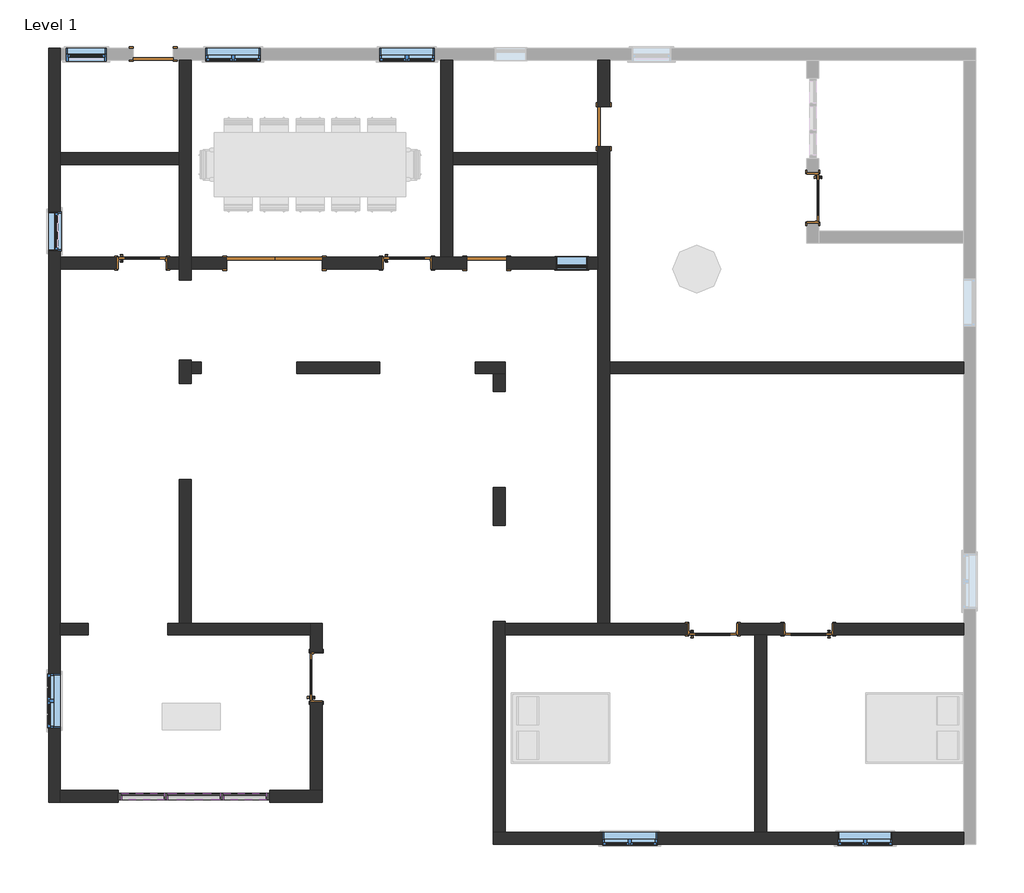
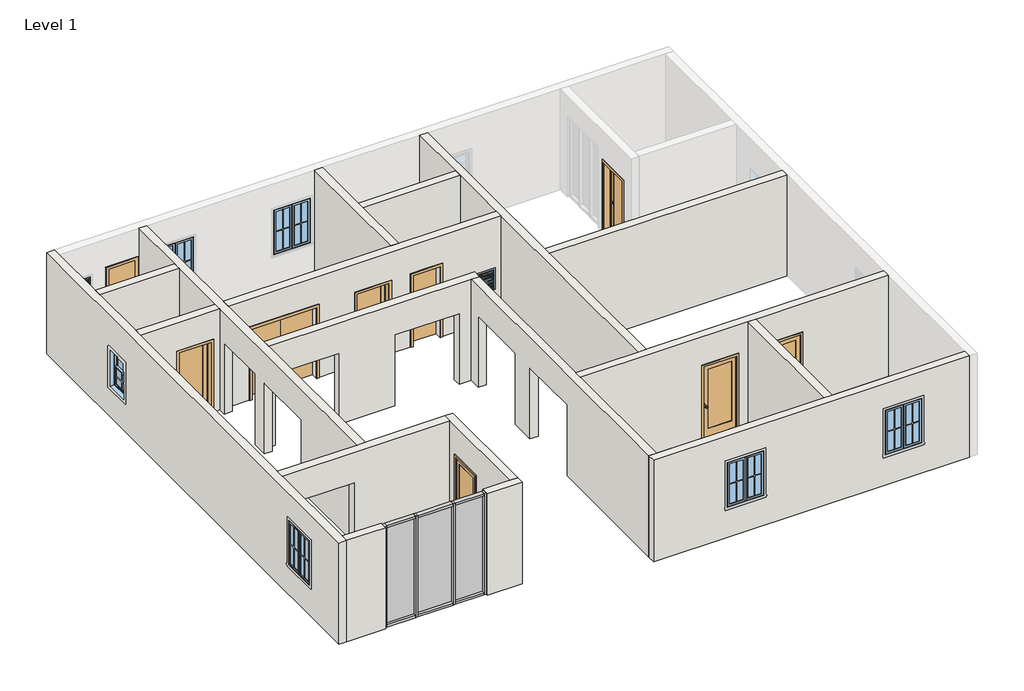
# One storey, part 1 of 2: 16 walls, 10 doors, 10 members, 8 windows, 3 plates.
"""IFC4 building model written with IfcOpenShell, lengths in millimetres."""

from ifc_helpers import new_model, si_unit, origin, origin_with_axes, place, context, project, spatial, polyline, outline, extrude, faceted_brep, transform, mapped, element, save
from components import door_963c5960, door_868ee8a9, door_3b97b8e7, door_5e1232af, member_c17f1be2, member_eaba9652, member_cfcad22e, member_3f395ae9, system_panel_glazed_52d31088, system_panel_glazed_62014e10, window_c95ebb39, window_d400040f, window_f2d8fef0

model = new_model("IFC4")

# Units and contexts
model_context = context("Model", 3, world=origin())
ifc_project = project(units=[si_unit("LENGTHUNIT", "METRE", prefix="MILLI")], contexts=[model_context])

# Site, building, storey
site = spatial("IfcSite", under=ifc_project)
building = spatial("IfcBuilding", under=site)
storey = spatial("IfcBuildingStorey", under=building, Name="Level 1", Elevation=0.0)

# Doors
placement = place(None, origin())
door_shape = door_963c5960(model_context)
element("IfcDoor", 1, ObjectType="Door-Double-Flush_Panel : 72\" x 84\"", at=placement, inside=storey, context=model_context, shape_type="MappedRepresentation", body=[
    mapped(door_shape, transform((-10733.2597103, 6532.3761524, 0.0), x_axis=(1.0, 0.0, 0.0), y_axis=(0.0, 1.0, 0.0), z_axis=(0.0, 0.0, 1.0))),
])
door_2_shape = door_868ee8a9(model_context)
element("IfcDoor", 2, ObjectType="Door-Interior-Single-1_Panel-Wood : 36\" x 84\"", at=placement, inside=storey, context=model_context, shape_type="MappedRepresentation", body=[
    mapped(door_2_shape, transform((-2354.8811947, -470.7808788, 0.0), x_axis=(1.0, 0.0, 0.0), y_axis=(0.0, 1.0, 0.0), z_axis=(0.0, 0.0, 1.0))),
])
door_3_shape = door_3b97b8e7(model_context)
element("IfcDoor", 3, ObjectType="Door-Interior-Single-1_Panel-Wood : 36\" x 84\"", at=placement, inside=storey, context=model_context, shape_type="MappedRepresentation", body=[
    mapped(door_3_shape, transform((-526.0811947, -470.7808788, 0.0), x_axis=(-1.0, 0.0, 0.0), y_axis=(0.0, -1.0, 0.0), z_axis=(0.0, 0.0, 1.0))),
])
element("IfcDoor", 4, ObjectType="Door-Interior-Single-1_Panel-Wood : 36\" x 84\"", at=placement, inside=storey, context=model_context, shape_type="MappedRepresentation", body=[
    mapped(door_3_shape, transform((-9943.6272884, -1382.0058788, 0.0), x_axis=(0.0, 1.0, 0.0), y_axis=(-1.0, 0.0, 0.0), z_axis=(0.0, 0.0, 1.0))),
])
element("IfcDoor", 5, ObjectType="Door-Interior-Single-1_Panel-Wood : 36\" x 84\"", at=placement, inside=storey, context=model_context, shape_type="MappedRepresentation", body=[
    mapped(door_3_shape, transform((-13264.0819759, 6535.5511524, 0.0), x_axis=(1.0, 0.0, 0.0), y_axis=(0.0, 1.0, 0.0), z_axis=(0.0, 0.0, 1.0))),
])
element("IfcDoor", 6, ObjectType="Door-Interior-Single-1_Panel-Wood : 36\" x 84\"", at=placement, inside=storey, context=model_context, shape_type="MappedRepresentation", body=[
    mapped(door_3_shape, transform((-8202.4374447, 6535.5511524, 0.0), x_axis=(1.0, 0.0, 0.0), y_axis=(0.0, 1.0, 0.0), z_axis=(0.0, 0.0, 1.0))),
])
element("IfcDoor", 7, ObjectType="Door-Interior-Single-1_Panel-Wood : 36\" x 84\"", at=placement, inside=storey, context=model_context, shape_type="MappedRepresentation", body=[
    mapped(door_3_shape, transform((-437.2804134, 7782.3835743, 0.0), x_axis=(0.0, -1.0, 0.0), y_axis=(1.0, 0.0, 0.0), z_axis=(0.0, 0.0, 1.0))),
])
door_4_shape = door_5e1232af(model_context)
element("IfcDoor", 8, ObjectType="Single-Flush : 30\" x 84\"", at=placement, inside=storey, context=model_context, shape_type="MappedRepresentation", body=[
    mapped(door_4_shape, transform((-13050.0671322, 10532.4792774, 0.0), x_axis=(1.0, 0.0, 0.0), y_axis=(0.0, 1.0, 0.0), z_axis=(0.0, 0.0, 1.0))),
])
element("IfcDoor", 9, ObjectType="Single-Flush : 30\" x 84\"", at=placement, inside=storey, context=model_context, shape_type="MappedRepresentation", body=[
    mapped(door_4_shape, transform((-4440.4593197, 9142.0277149, 0.0), x_axis=(0.0, -1.0, 0.0), y_axis=(1.0, 0.0, 0.0), z_axis=(0.0, 0.0, 1.0))),
])
element("IfcDoor", 10, ObjectType="Single-Flush : 30\" x 84\"", at=placement, inside=storey, context=model_context, shape_type="MappedRepresentation", body=[
    mapped(door_4_shape, transform((-6678.4374447, 6532.3761524, 0.0), x_axis=(-1.0, 0.0, 0.0), y_axis=(0.0, -1.0, 0.0), z_axis=(0.0, 0.0, 1.0))),
])

# Members
member_shape = member_c17f1be2(model_context)
element("IfcMember", 11, ObjectType="Rectangular Mullion : 2.5\" x 5\" rectangular", at=placement, inside=storey, context=model_context, shape_type="MappedRepresentation", body=[
    mapped(member_shape, transform((-10889.1819759, -3667.6090038, 3048.0), x_axis=(0.0, 0.0, 1.0), y_axis=(0.0, -1.0, 0.0), z_axis=(1.0, 0.0, 0.0))),
])
element("IfcMember", 12, ObjectType="Rectangular Mullion : 2.5\" x 5\" rectangular", at=placement, inside=storey, context=model_context, shape_type="MappedRepresentation", body=[
    mapped(member_shape, transform((-12838.6319759, -3667.6090038, 3048.0), x_axis=(0.0, 0.0, 1.0), y_axis=(0.0, -1.0, 0.0), z_axis=(1.0, 0.0, 0.0))),
])
element("IfcMember", 13, ObjectType="Rectangular Mullion : 2.5\" x 5\" rectangular", at=placement, inside=storey, context=model_context, shape_type="MappedRepresentation", body=[
    mapped(member_shape, transform((-13657.7819759, -3667.6090038, 0.0), x_axis=(0.0, 0.0, -1.0), y_axis=(0.0, -1.0, 0.0), z_axis=(-1.0, 0.0, 0.0))),
])
element("IfcMember", 14, ObjectType="Rectangular Mullion : 2.5\" x 5\" rectangular", at=placement, inside=storey, context=model_context, shape_type="MappedRepresentation", body=[
    mapped(member_shape, transform((-11708.3319759, -3667.6090038, 0.0), x_axis=(0.0, 0.0, -1.0), y_axis=(0.0, -1.0, 0.0), z_axis=(-1.0, 0.0, 0.0))),
])
member_2_shape = member_eaba9652(model_context)
element("IfcMember", 15, ObjectType="Rectangular Mullion : 2.5\" x 5\" rectangular", at=placement, inside=storey, context=model_context, shape_type="MappedRepresentation", body=[
    mapped(member_2_shape, transform((-12806.8819759, -3667.6090038, 0.0), x_axis=(1.0, 0.0, 0.0), y_axis=(0.0, -1.0, 0.0), z_axis=(0.0, 0.0, -1.0))),
])
element("IfcMember", 16, ObjectType="Rectangular Mullion : 2.5\" x 5\" rectangular", at=placement, inside=storey, context=model_context, shape_type="MappedRepresentation", body=[
    mapped(member_2_shape, transform((-11740.0819759, -3667.6090038, 0.0), x_axis=(1.0, 0.0, 0.0), y_axis=(0.0, -1.0, 0.0), z_axis=(0.0, 0.0, -1.0))),
])
member_3_shape = member_cfcad22e(model_context)
element("IfcMember", 17, ObjectType="Rectangular Mullion : 2.5\" x 5\" rectangular", at=placement, inside=storey, context=model_context, shape_type="MappedRepresentation", body=[
    mapped(member_3_shape, transform((-12775.1319759, -3667.6090038, 0.0), x_axis=(0.0, 0.0, -1.0), y_axis=(0.0, -1.0, 0.0), z_axis=(-1.0, 0.0, 0.0))),
])
element("IfcMember", 18, ObjectType="Rectangular Mullion : 2.5\" x 5\" rectangular", at=placement, inside=storey, context=model_context, shape_type="MappedRepresentation", body=[
    mapped(member_3_shape, transform((-11771.8319759, -3667.6090038, 3048.0), x_axis=(0.0, 0.0, 1.0), y_axis=(0.0, -1.0, 0.0), z_axis=(1.0, 0.0, 0.0))),
])
member_4_shape = member_3f395ae9(model_context)
element("IfcMember", 19, ObjectType="Rectangular Mullion : 2.5\" x 5\" rectangular", at=placement, inside=storey, context=model_context, shape_type="MappedRepresentation", body=[
    mapped(member_4_shape, transform((-13721.2819759, -3667.6090038, 3048.0), x_axis=(-1.0, 0.0, 0.0), y_axis=(0.0, -1.0, 0.0), z_axis=(0.0, 0.0, 1.0))),
])
element("IfcMember", 20, ObjectType="Rectangular Mullion : 2.5\" x 5\" rectangular", at=placement, inside=storey, context=model_context, shape_type="MappedRepresentation", body=[
    mapped(member_4_shape, transform((-10825.6819759, -3667.6090038, 0.0), x_axis=(1.0, 0.0, 0.0), y_axis=(0.0, -1.0, 0.0), z_axis=(0.0, 0.0, -1.0))),
])

# Plates
system_panel_glazed_shape = system_panel_glazed_52d31088(model_context)
element("IfcPlate", 21, ObjectType="System Panel : Glazed", at=placement, inside=storey, context=model_context, shape_type="MappedRepresentation", body=[
    mapped(system_panel_glazed_shape, transform((-13248.2069759, -3667.6090038, 63.5), x_axis=(1.0, 0.0, 0.0), y_axis=(0.0, 1.0, 0.0), z_axis=(0.0, 0.0, 1.0))),
])
element("IfcPlate", 22, ObjectType="System Panel : Glazed", at=placement, inside=storey, context=model_context, shape_type="MappedRepresentation", body=[
    mapped(system_panel_glazed_shape, transform((-11298.7569759, -3667.6090038, 63.5), x_axis=(1.0, 0.0, 0.0), y_axis=(0.0, 1.0, 0.0), z_axis=(0.0, 0.0, 1.0))),
])
system_panel_glazed_2_shape = system_panel_glazed_62014e10(model_context)
element("IfcPlate", 23, ObjectType="System Panel : Glazed", at=placement, inside=storey, context=model_context, shape_type="MappedRepresentation", body=[
    mapped(system_panel_glazed_2_shape, transform((-12273.4819759, -3667.6090038, 63.5), x_axis=(1.0, 0.0, 0.0), y_axis=(0.0, 1.0, 0.0), z_axis=(0.0, 0.0, 1.0))),
])

# Walls
element("IfcWall", 24, ObjectType="9\" wall", at=placement, inside=storey, context=model_context, shape_type="Brep", body=[
    faceted_brep([(-15054.7819759, 10646.7792774, 0.0), (-15054.7819759, -3781.9090038, 0.0), (-15054.7819759, -3781.9090038, 3048.0), (-15054.7819759, 10646.7792774, 3048.0), (-15054.7819759, -1318.5058788, 2260.6), (-15054.7819759, -2359.9058788, 2260.6), (-15054.7819759, -2359.9058788, 914.4), (-15054.7819759, -1318.5058788, 914.4), (-15054.7819759, 7522.9761524, 2082.8), (-15054.7819759, 6760.9761524, 2082.8), (-15054.7819759, 6760.9761524, 914.4), (-15054.7819759, 7522.9761524, 914.4), (-14826.1819759, 10646.7792774, 0.0), (-14826.1819759, 10646.7792774, 3048.0), (-14826.1819759, 10418.1792774, 3048.0), (-14826.1819759, 8646.6284962, 3048.0), (-14826.1819759, 8418.0284962, 3048.0), (-14826.1819759, 6646.6761524, 3048.0), (-14826.1819759, 6418.0761524, 3048.0), (-14826.1819759, -353.3058788, 3048.0), (-14826.1819759, -581.9058788, 3048.0), (-14826.1819759, -3553.3090038, 3048.0), (-14826.1819759, -3781.9090038, 3048.0), (-14826.1819759, -3781.9090038, 0.0), (-14826.1819759, -3553.3090038, 0.0), (-14826.1819759, -581.9058788, 0.0), (-14826.1819759, -353.3058788, 0.0), (-14826.1819759, 6418.0761524, 0.0), (-14826.1819759, 6646.6761524, 0.0), (-14826.1819759, 8418.0284962, 0.0), (-14826.1819759, 8646.6284962, 0.0), (-14826.1819759, 10418.1792774, 0.0), (-14826.1819759, -1318.5058788, 2260.6), (-14826.1819759, -1318.5058788, 914.4), (-14826.1819759, -2359.9058788, 914.4), (-14826.1819759, -2359.9058788, 2260.6), (-14826.1819759, 7522.9761524, 2082.8), (-14826.1819759, 7522.9761524, 914.4), (-14826.1819759, 6760.9761524, 914.4), (-14826.1819759, 6760.9761524, 2082.8)], [[[0, 1, 2, 3], [4, 5, 6, 7], [8, 9, 10, 11]], [[12, 13, 14, 15, 16, 17, 18, 19, 20, 21, 22, 23, 24, 25, 26, 27, 28, 29, 30, 31], [32, 33, 34, 35], [36, 37, 38, 39]], [[1, 0, 12, 31, 30, 29, 28, 27, 26, 25, 24, 23]], [[3, 2, 22, 21, 20, 19, 18, 17, 16, 15, 14, 13]], [[2, 1, 23, 22]], [[0, 3, 13, 12]], [[33, 32, 4, 7]], [[34, 33, 7, 6]], [[35, 34, 6, 5]], [[32, 35, 5, 4]], [[37, 36, 8, 11]], [[38, 37, 11, 10]], [[39, 38, 10, 9]], [[36, 39, 9, 8]]]),
])
element("IfcWall", 25, ObjectType="9\" wall", at=placement, inside=storey, context=model_context, shape_type="Brep", body=[
    faceted_brep([(-14826.1819759, -3781.9090038, 3048.0), (-14826.1819759, -3781.9090038, 0.0), (-13721.2819759, -3781.9090038, 0.0), (-13721.2819759, -3781.9090038, 3048.0), (-14826.1819759, -3553.3090038, 0.0), (-14826.1819759, -3553.3090038, 3048.0), (-13721.2819759, -3553.3090038, 3048.0), (-13721.2819759, -3553.3090038, 0.0)], [[[0, 1, 2, 3]], [[4, 5, 6, 7]], [[1, 4, 7, 2]], [[5, 0, 3, 6]], [[1, 0, 5, 4]], [[3, 2, 7, 6]]]),
    faceted_brep([(-9826.1522884, -3781.9090038, 0.0), (-9826.1522884, -3781.9090038, 3048.0), (-10825.6819759, -3781.9090038, 3048.0), (-10825.6819759, -3781.9090038, 0.0), (-9826.1522884, -3553.3090038, 3048.0), (-9826.1522884, -3553.3090038, 0.0), (-10054.7522884, -3553.3090038, 0.0), (-10825.6819759, -3553.3090038, 0.0), (-10825.6819759, -3553.3090038, 3048.0), (-10054.7522884, -3553.3090038, 3048.0)], [[[0, 1, 2, 3]], [[4, 5, 6, 7, 8, 9]], [[5, 0, 3, 7, 6]], [[1, 4, 9, 8, 2]], [[1, 0, 5, 4]], [[3, 2, 8, 7]]]),
])
element("IfcWall", 26, ObjectType="9\" wall", at=placement, inside=storey, context=model_context, shape_type="Brep", body=[
    faceted_brep([(-9826.1522884, -353.3058788, 3048.0), (-9826.1522884, -3553.3090038, 3048.0), (-9826.1522884, -3553.3090038, 0.0), (-9826.1522884, -1864.6058788, 0.0), (-9826.1522884, -1864.6058788, 2159.0), (-9826.1522884, -899.4058788, 2159.0), (-9826.1522884, -899.4058788, 0.0), (-9826.1522884, -353.3058788, 0.0), (-10054.7522884, -3553.3090038, 3048.0), (-10054.7522884, -581.9058788, 3048.0), (-10054.7522884, -353.3058788, 3048.0), (-10054.7522884, -353.3058788, 0.0), (-10054.7522884, -581.9058788, 0.0), (-10054.7522884, -899.4058788, 0.0), (-10054.7522884, -899.4058788, 2159.0), (-10054.7522884, -1864.6058788, 2159.0), (-10054.7522884, -1864.6058788, 0.0), (-10054.7522884, -3553.3090038, 0.0)], [[[0, 1, 2, 3, 4, 5, 6, 7]], [[8, 9, 10, 11, 12, 13, 14, 15, 16, 17]], [[2, 17, 16, 3]], [[11, 7, 6, 13, 12]], [[1, 0, 10, 9, 8]], [[2, 1, 8, 17]], [[0, 7, 11, 10]], [[5, 14, 13, 6]], [[14, 5, 4, 15]], [[15, 4, 3, 16]]]),
])
element("IfcWall", 27, ObjectType="9\" wall", at=placement, inside=storey, context=model_context, shape_type="Brep", body=[
    faceted_brep([(-14300.0745541, -353.3058788, 2133.6), (-14300.0745541, -353.3058788, 0.0), (-14826.1819759, -353.3058788, 0.0), (-14826.1819759, -353.3058788, 3048.0), (-12554.7671322, -353.3058788, 3048.0), (-12326.1671322, -353.3058788, 3048.0), (-10054.7522884, -353.3058788, 3048.0), (-10054.7522884, -353.3058788, 0.0), (-12326.1671322, -353.3058788, 0.0), (-12554.7671322, -353.3058788, 0.0), (-12776.0745541, -353.3058788, 0.0), (-12776.0745541, -353.3058788, 2133.6), (-14826.1819759, -581.9058788, 0.0), (-14300.0745541, -581.9058788, 0.0), (-14300.0745541, -581.9058788, 2133.6), (-12776.0745541, -581.9058788, 2133.6), (-12776.0745541, -581.9058788, 0.0), (-10054.7522884, -581.9058788, 0.0), (-10054.7522884, -581.9058788, 3048.0), (-14826.1819759, -581.9058788, 3048.0)], [[[0, 1, 2, 3, 4, 5, 6, 7, 8, 9, 10, 11]], [[12, 13, 14, 15, 16, 17, 18, 19]], [[2, 1, 13, 12]], [[10, 9, 8, 7, 17, 16]], [[6, 5, 4, 3, 19, 18]], [[7, 6, 18, 17]], [[3, 2, 12, 19]], [[16, 15, 11, 10]], [[14, 13, 1, 0]], [[15, 14, 0, 11]]]),
])
element("IfcWall", 28, ObjectType="9\" wall", at=placement, inside=storey, context=model_context, shape_type="Brep", body=[
    faceted_brep([(-12326.1671322, -353.3058788, 0.0), (-12326.1671322, 2398.8238087, 0.0), (-12326.1671322, 2398.8238087, 2133.6), (-12326.1671322, 4227.6238087, 2133.6), (-12326.1671322, 4227.6238087, 0.0), (-12326.1671322, 4418.1238087, 0.0), (-12326.1671322, 4646.7238087, 0.0), (-12326.1671322, 4684.8238087, 0.0), (-12326.1671322, 4684.8238087, 2133.6), (-12326.1671322, 6208.8238087, 2133.6), (-12326.1671322, 6208.8238087, 0.0), (-12326.1671322, 6418.0761524, 0.0), (-12326.1671322, 6646.6761524, 0.0), (-12326.1671322, 10418.1792774, 0.0), (-12326.1671322, 10418.1792774, 3048.0), (-12326.1671322, 6646.6761524, 3048.0), (-12326.1671322, 6418.0761524, 3048.0), (-12326.1671322, 4646.7238087, 3048.0), (-12326.1671322, 4418.1238087, 3048.0), (-12326.1671322, -353.3058788, 3048.0), (-12554.7671322, 2398.8238087, 2133.6), (-12554.7671322, 2398.8238087, 0.0), (-12554.7671322, -353.3058788, 0.0), (-12554.7671322, -353.3058788, 3048.0), (-12554.7671322, 6418.0761524, 3048.0), (-12554.7671322, 6646.6761524, 3048.0), (-12554.7671322, 8418.0284962, 3048.0), (-12554.7671322, 8646.6284962, 3048.0), (-12554.7671322, 10418.1792774, 3048.0), (-12554.7671322, 10418.1792774, 0.0), (-12554.7671322, 8646.6284962, 0.0), (-12554.7671322, 8418.0284962, 0.0), (-12554.7671322, 6646.6761524, 0.0), (-12554.7671322, 6418.0761524, 0.0), (-12554.7671322, 6208.8238087, 0.0), (-12554.7671322, 6208.8238087, 2133.6), (-12554.7671322, 4684.8238087, 2133.6), (-12554.7671322, 4684.8238087, 0.0), (-12554.7671322, 4227.6238087, 0.0), (-12554.7671322, 4227.6238087, 2133.6)], [[[0, 1, 2, 3, 4, 5, 6, 7, 8, 9, 10, 11, 12, 13, 14, 15, 16, 17, 18, 19]], [[20, 21, 22, 23, 24, 25, 26, 27, 28, 29, 30, 31, 32, 33, 34, 35, 36, 37, 38, 39]], [[13, 12, 11, 10, 34, 33, 32, 31, 30, 29]], [[38, 37, 7, 6, 5, 4]], [[22, 21, 1, 0]], [[19, 18, 17, 16, 15, 14, 28, 27, 26, 25, 24, 23]], [[0, 19, 23, 22]], [[14, 13, 29, 28]], [[37, 36, 8, 7]], [[35, 34, 10, 9]], [[36, 35, 9, 8]], [[4, 3, 39, 38]], [[2, 1, 21, 20]], [[3, 2, 20, 39]]]),
])
element("IfcWall", 29, ObjectType="9\" wall", at=placement, inside=storey, context=model_context, shape_type="Brep", body=[
    faceted_brep([(2445.2227116, -4353.3097851, 0.0), (-1326.1811947, -4353.3097851, 0.0), (-1554.7811947, -4353.3097851, 0.0), (-6326.1116634, -4353.3097851, 0.0), (-6554.7116634, -4353.3097851, 0.0), (-6554.7116634, -4353.3097851, 3048.0), (-6326.1116634, -4353.3097851, 3048.0), (-1554.7811947, -4353.3097851, 3048.0), (-1326.1811947, -4353.3097851, 3048.0), (2445.2227116, -4353.3097851, 3048.0), (-4461.1464291, -4353.3097851, 2260.6), (-4461.1464291, -4353.3097851, 914.4), (-3419.7464291, -4353.3097851, 914.4), (-3419.7464291, -4353.3097851, 2260.6), (38.8207584, -4353.3097851, 2260.6), (38.8207584, -4353.3097851, 914.4), (1080.2207584, -4353.3097851, 914.4), (1080.2207584, -4353.3097851, 2260.6), (2445.2227116, -4581.9097851, 0.0), (2445.2227116, -4581.9097851, 3048.0), (-6554.7116634, -4581.9097851, 3048.0), (-6554.7116634, -4581.9097851, 0.0), (-4461.1464291, -4581.9097851, 2260.6), (-3419.7464291, -4581.9097851, 2260.6), (-3419.7464291, -4581.9097851, 914.4), (-4461.1464291, -4581.9097851, 914.4), (38.8207584, -4581.9097851, 2260.6), (1080.2207584, -4581.9097851, 2260.6), (1080.2207584, -4581.9097851, 914.4), (38.8207584, -4581.9097851, 914.4)], [[[0, 1, 2, 3, 4, 5, 6, 7, 8, 9], [10, 11, 12, 13], [14, 15, 16, 17]], [[18, 19, 20, 21], [22, 23, 24, 25], [26, 27, 28, 29]], [[4, 3, 2, 1, 0, 18, 21]], [[9, 8, 7, 6, 5, 20, 19]], [[0, 9, 19, 18]], [[5, 4, 21, 20]], [[11, 10, 22, 25]], [[12, 11, 25, 24]], [[13, 12, 24, 23]], [[10, 13, 23, 22]], [[15, 14, 26, 29]], [[16, 15, 29, 28]], [[17, 16, 28, 27]], [[14, 17, 27, 26]]]),
])
element("IfcWall", 30, ObjectType="9\" wall", at=placement, inside=storey, context=model_context, shape_type="Brep", body=[
    faceted_brep([(-6326.1116634, -4353.3097851, 0.0), (-6326.1116634, -581.9058788, 0.0), (-6326.1116634, -353.3058788, 0.0), (-6326.1116634, -315.2058788, 0.0), (-6326.1116634, -315.2058788, 2133.6), (-6326.1116634, 1513.5941212, 2133.6), (-6326.1116634, 1513.5941212, 0.0), (-6326.1116634, 2246.4238087, 0.0), (-6326.1116634, 2246.4238087, 2133.6), (-6326.1116634, 4075.2238087, 2133.6), (-6326.1116634, 4075.2238087, 0.0), (-6326.1116634, 4418.1238087, 0.0), (-6326.1116634, 4418.1238087, 3048.0), (-6326.1116634, -353.3058788, 3048.0), (-6326.1116634, -581.9058788, 3048.0), (-6326.1116634, -4353.3097851, 3048.0), (-6554.7116634, -315.2058788, 2133.6), (-6554.7116634, -315.2058788, 0.0), (-6554.7116634, -4353.3097851, 0.0), (-6554.7116634, -4353.3097851, 3048.0), (-6554.7116634, 4418.1238087, 3048.0), (-6554.7116634, 4418.1238087, 0.0), (-6554.7116634, 4075.2238087, 0.0), (-6554.7116634, 4075.2238087, 2133.6), (-6554.7116634, 2246.4238087, 2133.6), (-6554.7116634, 2246.4238087, 0.0), (-6554.7116634, 1513.5941212, 0.0), (-6554.7116634, 1513.5941212, 2133.6)], [[[0, 1, 2, 3, 4, 5, 6, 7, 8, 9, 10, 11, 12, 13, 14, 15]], [[16, 17, 18, 19, 20, 21, 22, 23, 24, 25, 26, 27]], [[11, 10, 22, 21]], [[26, 25, 7, 6]], [[18, 17, 3, 2, 1, 0]], [[15, 14, 13, 12, 20, 19]], [[0, 15, 19, 18]], [[12, 11, 21, 20]], [[25, 24, 8, 7]], [[23, 22, 10, 9]], [[24, 23, 9, 8]], [[6, 5, 27, 26]], [[4, 3, 17, 16]], [[5, 4, 16, 27]]]),
])
element("IfcWall", 31, ObjectType="9\" wall", at=placement, inside=storey, context=model_context, shape_type="Brep", body=[
    faceted_brep([(2445.2227116, -581.9058788, 3048.0), (-1326.1811947, -581.9058788, 3048.0), (-1554.7811947, -581.9058788, 3048.0), (-6326.1116634, -581.9058788, 3048.0), (-6326.1116634, -581.9058788, 0.0), (-2837.4811947, -581.9058788, 0.0), (-2837.4811947, -581.9058788, 2159.0), (-1872.2811947, -581.9058788, 2159.0), (-1872.2811947, -581.9058788, 0.0), (-1554.7811947, -581.9058788, 0.0), (-1326.1811947, -581.9058788, 0.0), (-1008.6811947, -581.9058788, 0.0), (-1008.6811947, -581.9058788, 2159.0), (-43.4811947, -581.9058788, 2159.0), (-43.4811947, -581.9058788, 0.0), (2445.2227116, -581.9058788, 0.0), (-6326.1116634, -353.3058788, 3048.0), (-4554.7593197, -353.3058788, 3048.0), (-4326.1593197, -353.3058788, 3048.0), (2445.2227116, -353.3058788, 3048.0), (2445.2227116, -353.3058788, 0.0), (-43.4811947, -353.3058788, 0.0), (-43.4811947, -353.3058788, 2159.0), (-1008.6811947, -353.3058788, 2159.0), (-1008.6811947, -353.3058788, 0.0), (-1872.2811947, -353.3058788, 0.0), (-1872.2811947, -353.3058788, 2159.0), (-2837.4811947, -353.3058788, 2159.0), (-2837.4811947, -353.3058788, 0.0), (-4326.1593197, -353.3058788, 0.0), (-4554.7593197, -353.3058788, 0.0), (-6326.1116634, -353.3058788, 0.0)], [[[0, 1, 2, 3, 4, 5, 6, 7, 8, 9, 10, 11, 12, 13, 14, 15]], [[16, 17, 18, 19, 20, 21, 22, 23, 24, 25, 26, 27, 28, 29, 30, 31]], [[20, 15, 14, 21]], [[4, 31, 30, 29, 28, 5]], [[8, 25, 24, 11, 10, 9]], [[3, 2, 1, 0, 19, 18, 17, 16]], [[0, 15, 20, 19]], [[4, 3, 16, 31]], [[7, 26, 25, 8]], [[26, 7, 6, 27]], [[27, 6, 5, 28]], [[23, 12, 11, 24]], [[12, 23, 22, 13]], [[13, 22, 21, 14]]]),
])
element("IfcWall", 32, ObjectType="9\" wall", at=placement, inside=storey, context=model_context, shape_type="Brep", body=[
    faceted_brep([(-4326.1593197, -353.3058788, 0.0), (-4326.1593197, 4418.1238087, 0.0), (-4326.1593197, 4646.7238087, 0.0), (-4326.1593197, 8761.0277149, 0.0), (-4326.1593197, 8761.0277149, 2133.6), (-4326.1593197, 9523.0277149, 2133.6), (-4326.1593197, 9523.0277149, 0.0), (-4326.1593197, 10418.1792774, 0.0), (-4326.1593197, 10418.1792774, 3048.0), (-4326.1593197, 4646.7238087, 3048.0), (-4326.1593197, 4418.1238087, 3048.0), (-4326.1593197, -353.3058788, 3048.0), (-4554.7593197, 8761.0277149, 2133.6), (-4554.7593197, 8761.0277149, 0.0), (-4554.7593197, 8646.7277149, 0.0), (-4554.7593197, 8418.1277149, 0.0), (-4554.7593197, 6646.6761524, 0.0), (-4554.7593197, 6418.0761524, 0.0), (-4554.7593197, -353.3058788, 0.0), (-4554.7593197, -353.3058788, 3048.0), (-4554.7593197, 6418.0761524, 3048.0), (-4554.7593197, 6646.6761524, 3048.0), (-4554.7593197, 8418.1277149, 3048.0), (-4554.7593197, 8646.7277149, 3048.0), (-4554.7593197, 10418.1792774, 3048.0), (-4554.7593197, 10418.1792774, 0.0), (-4554.7593197, 9523.0277149, 0.0), (-4554.7593197, 9523.0277149, 2133.6)], [[[0, 1, 2, 3, 4, 5, 6, 7, 8, 9, 10, 11]], [[12, 13, 14, 15, 16, 17, 18, 19, 20, 21, 22, 23, 24, 25, 26, 27]], [[26, 25, 7, 6]], [[18, 17, 16, 15, 14, 13, 3, 2, 1, 0]], [[11, 10, 9, 8, 24, 23, 22, 21, 20, 19]], [[0, 11, 19, 18]], [[8, 7, 25, 24]], [[4, 3, 13, 12]], [[5, 4, 12, 27]], [[6, 5, 27, 26]]]),
])
element("IfcWall", 33, ObjectType="9\" wall", at=placement, inside=storey, context=model_context, shape_type="SweptSolid", body=[
    extrude(outline(polyline([(-4326.1593197, 4646.7238087), (2445.2227116, 4646.7238087), (2445.2227116, 4418.1238087), (-4326.1593197, 4418.1238087), (-4326.1593197, 4646.7238087)])), origin_with_axes(), (0.0, 0.0, 1.0), 3048.0),
])
element("IfcWall", 34, ObjectType="9\" wall", at=placement, inside=storey, context=model_context, shape_type="SweptSolid", body=[
    extrude(outline(polyline([(-1326.1811947, -581.9058788), (-1326.1811947, -4353.3097851), (-1554.7811947, -4353.3097851), (-1554.7811947, -581.9058788), (-1326.1811947, -581.9058788)])), origin_with_axes(), (0.0, 0.0, 1.0), 3048.0),
])
element("IfcWall", 35, ObjectType="9\" wall", at=placement, inside=storey, context=model_context, shape_type="Brep", body=[
    faceted_brep([(-10306.8671322, 4418.1238087, 0.0), (-8726.4116634, 4418.1238087, 0.0), (-8726.4116634, 4418.1238087, 2133.6), (-6897.6116634, 4418.1238087, 2133.6), (-6897.6116634, 4418.1238087, 0.0), (-6554.7116634, 4418.1238087, 0.0), (-6326.1116634, 4418.1238087, 0.0), (-6326.1116634, 4418.1238087, 3048.0), (-6554.7116634, 4418.1238087, 3048.0), (-12326.1671322, 4418.1238087, 3048.0), (-12326.1671322, 4418.1238087, 0.0), (-12135.6671322, 4418.1238087, 0.0), (-12135.6671322, 4418.1238087, 2133.6), (-10306.8671322, 4418.1238087, 2133.6), (-8726.4116634, 4646.7238087, 2133.6), (-8726.4116634, 4646.7238087, 0.0), (-10306.8671322, 4646.7238087, 0.0), (-10306.8671322, 4646.7238087, 2133.6), (-12135.6671322, 4646.7238087, 2133.6), (-12135.6671322, 4646.7238087, 0.0), (-12326.1671322, 4646.7238087, 0.0), (-12326.1671322, 4646.7238087, 3048.0), (-6326.1116634, 4646.7238087, 3048.0), (-6326.1116634, 4646.7238087, 0.0), (-6897.6116634, 4646.7238087, 0.0), (-6897.6116634, 4646.7238087, 2133.6)], [[[0, 1, 2, 3, 4, 5, 6, 7, 8, 9, 10, 11, 12, 13]], [[14, 15, 16, 17, 18, 19, 20, 21, 22, 23, 24, 25]], [[11, 10, 20, 19]], [[24, 23, 6, 5, 4]], [[16, 15, 1, 0]], [[9, 8, 7, 22, 21]], [[10, 9, 21, 20]], [[7, 6, 23, 22]], [[19, 18, 12, 11]], [[17, 16, 0, 13]], [[18, 17, 13, 12]], [[4, 3, 25, 24]], [[2, 1, 15, 14]], [[3, 2, 14, 25]]]),
])
element("IfcWall", 36, ObjectType="9\" wall", at=placement, inside=storey, context=model_context, shape_type="Brep", body=[
    faceted_brep([(-14826.1819759, 6418.0761524, 3048.0), (-14826.1819759, 6418.0761524, 0.0), (-13746.6819759, 6418.0761524, 0.0), (-13746.6819759, 6418.0761524, 2159.0), (-12781.4819759, 6418.0761524, 2159.0), (-12781.4819759, 6418.0761524, 0.0), (-12554.7671322, 6418.0761524, 0.0), (-12554.7671322, 6418.0761524, 3048.0), (-14826.1819759, 6646.6761524, 0.0), (-14826.1819759, 6646.6761524, 3048.0), (-12554.7671322, 6646.6761524, 3048.0), (-12554.7671322, 6646.6761524, 0.0), (-12781.4819759, 6646.6761524, 0.0), (-12781.4819759, 6646.6761524, 2159.0), (-13746.6819759, 6646.6761524, 2159.0), (-13746.6819759, 6646.6761524, 0.0)], [[[0, 1, 2, 3, 4, 5, 6, 7]], [[8, 9, 10, 11, 12, 13, 14, 15]], [[1, 8, 15, 2]], [[5, 12, 11, 6]], [[9, 0, 7, 10]], [[1, 0, 9, 8]], [[7, 6, 11, 10]], [[4, 13, 12, 5]], [[13, 4, 3, 14]], [[14, 3, 2, 15]]]),
    faceted_brep([(-4554.7593197, 6418.0761524, 0.0), (-4554.7593197, 6418.0761524, 3048.0), (-12326.1671322, 6418.0761524, 3048.0), (-12326.1671322, 6418.0761524, 0.0), (-11647.6597103, 6418.0761524, 0.0), (-11647.6597103, 6418.0761524, 2133.6), (-9818.8597103, 6418.0761524, 2133.6), (-9818.8597103, 6418.0761524, 0.0), (-8685.0374447, 6418.0761524, 0.0), (-8685.0374447, 6418.0761524, 2159.0), (-7719.8374447, 6418.0761524, 2159.0), (-7719.8374447, 6418.0761524, 0.0), (-7059.4374447, 6418.0761524, 0.0), (-7059.4374447, 6418.0761524, 2133.6), (-6297.4374447, 6418.0761524, 2133.6), (-6297.4374447, 6418.0761524, 0.0), (-4745.2593197, 6418.0761524, 1524.0), (-4745.2593197, 6418.0761524, 914.4), (-5354.8593197, 6418.0761524, 914.4), (-5354.8593197, 6418.0761524, 1524.0), (-4554.7593197, 6646.6761524, 3048.0), (-4554.7593197, 6646.6761524, 0.0), (-6297.4374447, 6646.6761524, 0.0), (-6297.4374447, 6646.6761524, 2133.6), (-7059.4374447, 6646.6761524, 2133.6), (-7059.4374447, 6646.6761524, 0.0), (-7326.1374447, 6646.6761524, 0.0), (-7554.7374447, 6646.6761524, 0.0), (-7719.8374447, 6646.6761524, 0.0), (-7719.8374447, 6646.6761524, 2159.0), (-8685.0374447, 6646.6761524, 2159.0), (-8685.0374447, 6646.6761524, 0.0), (-9818.8597103, 6646.6761524, 0.0), (-9818.8597103, 6646.6761524, 2133.6), (-11647.6597103, 6646.6761524, 2133.6), (-11647.6597103, 6646.6761524, 0.0), (-12326.1671322, 6646.6761524, 0.0), (-12326.1671322, 6646.6761524, 3048.0), (-7554.7374447, 6646.6761524, 3048.0), (-7326.1374447, 6646.6761524, 3048.0), (-4745.2593197, 6646.6761524, 914.4), (-4745.2593197, 6646.6761524, 1524.0), (-5354.8593197, 6646.6761524, 1524.0), (-5354.8593197, 6646.6761524, 914.4)], [[[0, 1, 2, 3, 4, 5, 6, 7, 8, 9, 10, 11, 12, 13, 14, 15], [16, 17, 18, 19]], [[20, 21, 22, 23, 24, 25, 26, 27, 28, 29, 30, 31, 32, 33, 34, 35, 36, 37, 38, 39], [40, 41, 42, 43]], [[21, 0, 15, 22]], [[11, 28, 27, 26, 25, 12]], [[31, 8, 7, 32]], [[35, 4, 3, 36]], [[1, 20, 39, 38, 37, 2]], [[1, 0, 21, 20]], [[3, 2, 37, 36]], [[10, 29, 28, 11]], [[29, 10, 9, 30]], [[30, 9, 8, 31]], [[6, 33, 32, 7]], [[33, 6, 5, 34]], [[34, 5, 4, 35]], [[17, 16, 41, 40]], [[18, 17, 40, 43]], [[19, 18, 43, 42]], [[16, 19, 42, 41]], [[13, 12, 25, 24]], [[14, 13, 24, 23]], [[15, 14, 23, 22]]]),
])
element("IfcWall", 37, ObjectType="9\" wall", at=placement, inside=storey, context=model_context, shape_type="Brep", body=[
    faceted_brep([(-7554.7374447, 10418.1792774, 0.0), (-7554.7374447, 6646.6761524, 0.0), (-7554.7374447, 6646.6761524, 3048.0), (-7554.7374447, 10418.1792774, 3048.0), (-7326.1374447, 10418.1792774, 0.0), (-7326.1374447, 10418.1792774, 3048.0), (-7326.1374447, 8646.7277149, 3048.0), (-7326.1374447, 8418.1277149, 3048.0), (-7326.1374447, 6646.6761524, 3048.0), (-7326.1374447, 6646.6761524, 0.0), (-7326.1374447, 8418.1277149, 0.0), (-7326.1374447, 8646.7277149, 0.0)], [[[0, 1, 2, 3]], [[4, 5, 6, 7, 8, 9, 10, 11]], [[1, 0, 4, 11, 10, 9]], [[3, 2, 8, 7, 6, 5]], [[0, 3, 5, 4]], [[2, 1, 9, 8]]]),
])
element("IfcWall", 38, ObjectType="9\" wall", at=placement, inside=storey, context=model_context, shape_type="SweptSolid", body=[
    extrude(outline(polyline([(-12554.7671322, 8418.0284962), (-14826.1819759, 8418.0284962), (-14826.1819759, 8646.6284962), (-12554.7671322, 8646.6284962), (-12554.7671322, 8418.0284962)])), origin_with_axes(), (0.0, 0.0, 1.0), 3048.0),
])
element("IfcWall", 39, ObjectType="9\" wall", at=placement, inside=storey, context=model_context, shape_type="SweptSolid", body=[
    extrude(outline(polyline([(-4554.7593197, 8418.1277149), (-7326.1374447, 8418.1277149), (-7326.1374447, 8646.7277149), (-4554.7593197, 8646.7277149), (-4554.7593197, 8418.1277149)])), origin_with_axes(), (0.0, 0.0, 1.0), 3048.0),
])

# Windows
window_shape = window_c95ebb39(model_context)
element("IfcWindow", 40, ObjectType="Window-Casement-Double : 41\" x 53\"", at=placement, inside=storey, context=model_context, shape_type="MappedRepresentation", body=[
    mapped(window_shape, transform((-3940.4464291, -4467.6097851, 0.0), x_axis=(-1.0, 0.0, 0.0), y_axis=(0.0, -1.0, 0.0), z_axis=(0.0, 0.0, 1.0))),
])
element("IfcWindow", 41, ObjectType="Window-Casement-Double : 41\" x 53\"", at=placement, inside=storey, context=model_context, shape_type="MappedRepresentation", body=[
    mapped(window_shape, transform((559.5207584, -4467.6097851, 0.0), x_axis=(-1.0, 0.0, 0.0), y_axis=(0.0, -1.0, 0.0), z_axis=(0.0, 0.0, 1.0))),
])
element("IfcWindow", 42, ObjectType="Window-Casement-Double : 41\" x 53\"", at=placement, inside=storey, context=model_context, shape_type="MappedRepresentation", body=[
    mapped(window_shape, transform((-14940.4819759, -1839.2058788, 0.0), x_axis=(0.0, 1.0, 0.0), y_axis=(-1.0, 0.0, 0.0), z_axis=(0.0, 0.0, 1.0))),
])
element("IfcWindow", 43, ObjectType="Window-Casement-Double : 41\" x 53\"", at=placement, inside=storey, context=model_context, shape_type="MappedRepresentation", body=[
    mapped(window_shape, transform((-11526.0671322, 10532.4792774, 0.0), x_axis=(-1.0, 0.0, 0.0), y_axis=(0.0, -1.0, 0.0), z_axis=(0.0, 0.0, 1.0))),
])
element("IfcWindow", 44, ObjectType="Window-Casement-Double : 41\" x 53\"", at=placement, inside=storey, context=model_context, shape_type="MappedRepresentation", body=[
    mapped(window_shape, transform((-8202.4374447, 10532.4792774, 0.0), x_axis=(-1.0, 0.0, 0.0), y_axis=(0.0, -1.0, 0.0), z_axis=(0.0, 0.0, 1.0))),
])
window_2_shape = window_d400040f(model_context)
element("IfcWindow", 45, ObjectType="Window-Double-Hung : 30\" x 46\"", at=placement, inside=storey, context=model_context, shape_type="MappedRepresentation", body=[
    mapped(window_2_shape, transform((-14940.4819759, 7141.9761524, 0.0), x_axis=(0.0, -1.0, 0.0), y_axis=(1.0, 0.0, 0.0), z_axis=(0.0, 0.0, 1.0))),
])
element("IfcWindow", 46, ObjectType="Window-Double-Hung : 30\" x 46\"", at=placement, inside=storey, context=model_context, shape_type="MappedRepresentation", body=[
    mapped(window_2_shape, transform((-14330.8819759, 10532.4792774, 0.0), x_axis=(-1.0, 0.0, 0.0), y_axis=(0.0, -1.0, 0.0), z_axis=(0.0, 0.0, 1.0))),
])
window_3_shape = window_f2d8fef0(model_context)
element("IfcWindow", 47, ObjectType="Window-Louvers : 24\" x 24\"", at=placement, inside=storey, context=model_context, shape_type="MappedRepresentation", body=[
    mapped(window_3_shape, transform((-5050.0593197, 6526.0261524, 0.0), x_axis=(-1.0, 0.0, 0.0), y_axis=(0.0, -1.0, 0.0), z_axis=(0.0, 0.0, 1.0))),
])

save(model, "model.ifc")

# Revit data of these elements
# Grids (mm)
#   "A": line (-14940.482, 13616.137) -> (-14940.482, -8053.993)
#   "2": line (-16643.163, -3667.609) -> (5253.481, -3667.609)
#   "D": line (-7440.437, 13616.137) -> (-7440.437, -8053.993)
#   "E": line (-6440.412, 13616.137) -> (-6440.412, -8053.993)
#   "B": line (-12440.467, 13616.137) -> (-12440.467, -8053.993)
#   "C": line (-9940.452, 13616.137) -> (-9940.452, -8053.993)
#   "8": line (-16643.163, 8532.328) -> (5253.481, 8532.328)
#   "F": line (-4440.459, 13616.137) -> (-4440.459, -8053.993)
#   "G": line (-1440.481, 13616.137) -> (-1440.481, -8053.993)
#   "H": line (-440.455, 13616.137) -> (-440.455, -8053.993)
#   "I": line (2559.523, 13616.137) -> (2559.523, -8053.993)
#   "1": line (-16643.163, -4467.61) -> (5253.481, -4467.61)
#   "3": line (-16643.163, -467.606) -> (5253.481, -467.606)
#   "6": line (-16643.163, 6532.376) -> (5253.481, 6532.376)
#   "4": line (-16643.163, 2032.409) -> (5253.481, 2032.409)
#   "5": line (-16643.163, 4532.424) -> (5253.481, 4532.424)
#   "7": line (-16643.163, 7032.439) -> (5253.481, 7032.439)
#   "9": line (-16643.163, 10532.479) -> (5253.481, 10532.479)
# Type "Door-Double-Flush_Panel : 72\" x 84\""
#   Type Mark = "16"
#   Construction Type Id = "DOOR"
#   Assembly Code = "C1020"
#   Analytic Construction = "Wooden"
#   Thickness = 0' - 2"
#   Thermal Resistance (R) = 2.5876 (h·ft²·°F)/BTU
#   Swing Angle [instance default] = 90.00°
#   Panel Width = 3' - 0"
#   Heat Transfer Coefficient (U) = 0.3865 BTU/(h·ft²·°F)
#   Height = 7' - 0"
#   Trim Projection Ext = 0' - 1"
#   Trim Projection Int = 0' - 1"
#   Trim Width = 0' - 3"
#   Width = 6' - 0"
#   Define Thermal Properties by = 1
#   Panel Material = Wood - Birch - Solid Stained Light Low Gloss
#   Trim Material = Paint - Sienna
#   Visual Light Transmittance = 0
#   Solar Heat Gain Coefficient = 0
#   Function = (empty or 0)
#   Wall Closure = (empty or 0)
# Type "Door-Interior-Single-1_Panel-Wood : 36\" x 84\""
#   Type Mark = "17"
#   Assembly Code = "C1020300"
#   Analytic Construction = "Wooden"
#   Top Rail = 0' - 4 11/16"
#   Thickness = 0' - 1 3/8"
#   Thermal Resistance (R) = 2.5876 (h·ft²·°F)/BTU
#   Swing Angle [instance default] = 90.00°
#   Stiles = 0' - 4 3/4"
#   Rough Width = 3' - 2"
#   Rough Height = 7' - 1"
#   Height = 7' - 0"
#   Width = 3' - 0"
#   Heat Transfer Coefficient (U) = 0.3865 BTU/(h·ft²·°F)
#   Bottom Rail = 0' - 9 1/8"
#   Trim Material = Cherry
#   Panel Material = Cherry
#   Frame Material = Cherry
#   Door Handle Material = Aluminum
#   Visual Light Transmittance = 0
#   Solar Heat Gain Coefficient = 0
#   Wall Closure = (empty or 0)
#   Function = (empty or 0)
# Type "Single-Flush : 30\" x 84\""
#   Type Mark = "4"
#   Construction Type Id = "MDOOR"
#   Assembly Code = "C1020"
#   Analytic Construction = "Metal"
#   Thickness = 0' - 2"
#   Heat Transfer Coefficient (U) = 0.651978 BTU/(h·ft²·°F)
#   Height = 7' - 0"
#   Trim Projection Ext = 0' - 1"
#   Trim Projection Int = 0' - 1"
#   Trim Width = 0' - 3"
#   Width = 2' - 6"
#   Define Thermal Properties by = 1
#   Define Thermal Properties by = 1
#   Door Material = Door - Panel
#   Frame Material = Door - Frame
#   Visual Light Transmittance = 0
#   Solar Heat Gain Coefficient = 0
#   Function = (empty or 0)
#   Wall Closure = (empty or 0)
# Type "Rectangular Mullion : 2.5\" x 5\" rectangular"
#   built-in parameter 1007304 = 0.416667 (stored number, unit not read)
#   built-in parameter 1007301 = 0.104167 (stored number, unit not read)
#   built-in parameter 1007300 = 0.104167 (stored number, unit not read)
# Type "System Panel : Glazed"
#   Construction Type Id = "GSP4R"
#   Analytic Construction = "1/8 in Pilkington single glazing"
#   Visual Light Transmittance = 0.9
#   Solar Heat Gain Coefficient = 0.86
#   Heat Transfer Coefficient (U) = 1.18115 BTU/(h·ft²·°F)
#   Define Thermal Properties by = 1
# Type "9\" wall"
#   Assembly Code = "B2010"
#   Layers, outside or top first: 0' - 9" no material (function 1)
# Type "Window-Casement-Double : 41\" x 53\""
#   Type Mark = "15"
#   Fire Rating = "0.5h"
#   Assembly Code = "B2020100"
#   Analytic Construction = "Double glazing - domestic"
#   Frame Extension [instance default] = 0' - 0 1/4"
#   Window Inset [instance default] = 0' - 0"
#   Wall Thickness [instance default] = 0' - 6"
#   Interior Wall Closure [instance default] = 0' - 2 1/4"
#   Half Width = 1' - 8 1/2"
#   Visual Light Transmittance = 0.81
#   Thermal Resistance (R) = 1.8146 (h·ft²·°F)/BTU
#   Solar Heat Gain Coefficient = 0.76
#   Rough Width = 3' - 5 1/2"
#   Rough Height = 4' - 5 1/2"
#   Height = 4' - 5"
#   Heat Transfer Coefficient (U) = 0.5511 BTU/(h·ft²·°F)
#   Exterior Wall Closure [instance default] = 0' - 1 1/4"
#   Extension Jamb [instance default] = 0' - 2 1/4"
#   Default Sill Height = 3' - 0"
#   Width = 3' - 5"
#   Define Thermal Properties by = 0
#   Muntin Visibility = yes
#   Interior Trim Visibility [instance default] = yes
#   Exterior Trim Visibility [instance default] = yes
#   Extension Jamb Visibility [instance default] = yes
#   Interior Trim Material = Wood - Stained
#   Muntin Pattern = Muntin Pattern_2x2 : Muntin Pattern_2x2
#   Interior Trim = Trim-Window-Interior-Flat : Picture Frame
#   Interior Frame Material = Wood - Stained
#   Glass Panel Material = Glass
#   Exterior Trim Material = Clad - White
#   Exterior Trim = Trim-Window-Exterior-Flat : with Sill
#   Exterior Frame Material = Clad - White
#   Wall Closure = (empty or 0)
# Type "Window-Double-Hung : 30\" x 46\""
#   Type Mark = "13"
#   Fire Rating = "0.5h"
#   Construction Type Id = "DG-DR"
#   Assembly Code = "B2020100"
#   Analytic Construction = "Double glazing - domestic"
#   Wall Thickness [instance default] = 0' - 6"
#   Window Inset [instance default] = 0' - 0"
#   Visual Light Transmittance = 0.81
#   Thermal Resistance (R) = 1.8146 (h·ft²·°F)/BTU
#   Solar Heat Gain Coefficient = 0.76
#   Muntin Width = 2' - 0"
#   Muntin Height = 1' - 7 1/8"
#   Interior Wall Closure [instance default] = 0' - 1 1/2"
#   Rough Width = 2' - 6 1/2"
#   Rough Height = 3' - 10 1/2"
#   Frame Extension [instance default] = 0' - 1 1/4"
#   Exterior Wall Closure [instance default] = 0' - 0 1/2"
#   Extension Jamb [instance default] = 0' - 1 1/2"
#   Heat Transfer Coefficient (U) = 0.5511 BTU/(h·ft²·°F)
#   Height = 3' - 10"
#   Width = 2' - 6"
#   Define Thermal Properties by = 1
#   Top Muntin Visibility = yes
#   Indicator Visibility [instance default] = yes
#   Extension Jamb Visibility [instance default] = yes
#   Interior Trim Visibility [instance default] = yes
#   Exterior Trim Visibility [instance default] = yes
#   Define Thermal Properties by = 1
#   Bottom Muntin Visibility = yes
#   Muntin Pattern = Muntin Pattern_2x2 : Muntin Pattern_2x2
#   Interior Trim Material = Wood - Stained
#   Interior Trim = Trim-Window-Interior-Flat : Picture Frame
#   Exterior Trim Material = Clad - White
#   Exterior Trim = Trim-Window-Exterior-Flat : with Sill
#   Glass Panel Material = Glass
#   Exterior Frame Material = Clad - White
#   Interior Frame Material = Wood - Stained
#   Wall Closure = (empty or 0)
# Type "Window-Louvers : 24\" x 24\""
#   Type Mark = "18"
#   Construction Type Id = "GSP4R"
#   Assembly Code = "B20"
#   Analytic Construction = "1/8 in Pilkington single glazing"
#   Visual Light Transmittance = 0.9
#   Thermal Resistance (R) = 1.53941 (h·ft²·°F)/BTU
#   Solar Heat Gain Coefficient = 0.78
#   Max Height = 1' - 11.74264"
#   Height = 2' - 0"
#   Heat Transfer Coefficient (U) = 0.6496 BTU/(h·ft²·°F)
#   Blade Width [instance default] = 1' - 10 1/2"
#   Blade Vertical Thickness = 0' - 0.35355"
#   Blade Thickness = 0' - 0 1/4"
#   Blade Spacing = 0' - 1 1/2"
#   Blade Height = 0' - 1.85355"
#   Blade Depth = 0' - 3"
#   Blade Angle = 45.00°
#   Default Sill Height = 3' - 0"
#   Trim Projection_Exterior = 0' - 0 1/2"
#   Trim Projection_Interior = 0' - 0 1/2"
#   Trim Width_Exterior = 0' - 1 1/2"
#   Trim Width_Interior = 0' - 1 1/2"
#   Width = 2' - 0"
#   Max Blade Count = 12
#   Define Thermal Properties by = 1
#   Blade Count = 12
#   Frame Material = Birch
#   Louver Material = Birch
#   Trim Exterior Material = Birch
#   Trim Interior Material = Birch
#   Wall Closure = (empty or 0)
# Element 1 (IfcDoor, "Door-Double-Flush_Panel : 72\" x 84\"")
#   Swing Angle = 90.00°
#   Phase Created = New Construction
#   Materials on its faces: "Paint - Sienna", "Wood - Birch - Solid Stained Light Low Gloss"
# Elements 2, 3, 4, 5, 6, 7 (IfcDoor, "Door-Interior-Single-1_Panel-Wood : 36\" x 84\"")
#   Swing Angle = 90.00°
#   Phase Created = New Construction
#   Materials on its faces: "Cherry", "Aluminum"
# Elements 8, 9, 10 (IfcDoor, "Single-Flush : 30\" x 84\"")
#   Phase Created = New Construction
#   Materials on its faces: "Door - Frame", "Door - Panel"
# Elements 11, 12, 13, 14, 15, 16, 17, 18, 19, 20 (IfcMember, "Rectangular Mullion : 2.5\" x 5\" rectangular")
#   Phase Created = New Construction
#   Materials on its faces: "Aluminum"
# Elements 21, 22, 23 (IfcPlate, "System Panel : Glazed")
#   Phase Created = New Construction
#   Materials on its faces: "Glass"
# Elements 24, 25, 26, 27, 28, 29, 30, 31, 32, 33, 34, 35, 36, 37, 38, 39 (IfcWall, "9\" wall")
#   Top Offset = 0' - 0"
#   Base Offset = 0' - 0"
#   wall height = 10' - 0"
#   Phase Created = New Construction
#   Base Constraint = Level 1
#   Top Constraint = Level 2
#   Materials on its faces: "Default Wall"
# Element 40 (IfcWindow, "Window-Casement-Double : 41\" x 53\"")
#   Mark = "2"
#   Window Inset = 0' - 0"
#   Interior Wall Closure = 0' - 2 1/4"
#   Frame Extension = 0' - 0 1/4"
#   Exterior Wall Closure = 0' - 1 1/4"
#   Interior Trim Visibility = yes
#   Exterior Trim Visibility = yes
#   Phase Created = New Construction
#   Materials on its faces: "Wood - Stained", "Glass", "Clad - White"
# Element 41 (IfcWindow, "Window-Casement-Double : 41\" x 53\"")
#   Mark = "3"
#   Window Inset = 0' - 0"
#   Interior Wall Closure = 0' - 2 1/4"
#   Frame Extension = 0' - 0 1/4"
#   Exterior Wall Closure = 0' - 1 1/4"
#   Interior Trim Visibility = yes
#   Exterior Trim Visibility = yes
#   Phase Created = New Construction
#   Materials on its faces: "Wood - Stained", "Glass", "Clad - White"
# Element 42 (IfcWindow, "Window-Casement-Double : 41\" x 53\"")
#   Mark = "5"
#   Window Inset = 0' - 0"
#   Interior Wall Closure = 0' - 2 1/4"
#   Frame Extension = 0' - 0 1/4"
#   Exterior Wall Closure = 0' - 1 1/4"
#   Interior Trim Visibility = yes
#   Exterior Trim Visibility = yes
#   Phase Created = New Construction
#   Materials on its faces: "Wood - Stained", "Glass", "Clad - White"
# Element 43 (IfcWindow, "Window-Casement-Double : 41\" x 53\"")
#   Mark = "6"
#   Window Inset = 0' - 0"
#   Interior Wall Closure = 0' - 2 1/4"
#   Frame Extension = 0' - 0 1/4"
#   Exterior Wall Closure = 0' - 1 1/4"
#   Interior Trim Visibility = yes
#   Exterior Trim Visibility = yes
#   Phase Created = New Construction
#   Materials on its faces: "Wood - Stained", "Glass", "Clad - White"
# Element 44 (IfcWindow, "Window-Casement-Double : 41\" x 53\"")
#   Mark = "7"
#   Window Inset = 0' - 0"
#   Interior Wall Closure = 0' - 2 1/4"
#   Frame Extension = 0' - 0 1/4"
#   Exterior Wall Closure = 0' - 1 1/4"
#   Interior Trim Visibility = yes
#   Exterior Trim Visibility = yes
#   Phase Created = New Construction
#   Materials on its faces: "Wood - Stained", "Glass", "Clad - White"
# Element 45 (IfcWindow, "Window-Double-Hung : 30\" x 46\"")
#   Mark = "10"
#   Window Inset = 0' - 0"
#   Interior Wall Closure = 0' - 1 1/2"
#   Frame Extension = 0' - 1 1/4"
#   Exterior Wall Closure = 0' - 0 1/2"
#   Interior Trim Visibility = yes
#   Indicator Visibility = yes
#   Exterior Trim Visibility = yes
#   Phase Created = New Construction
#   Materials on its faces: "Wood - Stained", "Glass", "Clad - White"
# Element 46 (IfcWindow, "Window-Double-Hung : 30\" x 46\"")
#   Mark = "11"
#   Window Inset = 0' - 0"
#   Interior Wall Closure = 0' - 1 1/2"
#   Frame Extension = 0' - 1 1/4"
#   Exterior Wall Closure = 0' - 0 1/2"
#   Interior Trim Visibility = yes
#   Indicator Visibility = yes
#   Exterior Trim Visibility = yes
#   Phase Created = New Construction
#   Materials on its faces: "Wood - Stained", "Glass", "Clad - White"
# Element 47 (IfcWindow, "Window-Louvers : 24\" x 24\"")
#   Mark = "8"
#   Blade Width = 1' - 10 1/2"
#   Phase Created = New Construction
#   Materials on its faces: "Birch"
# Materials
#   "Wood - Birch - Solid Stained Light Low Gloss": class "Wood", colour RGB 210 159 95, transparency 0, Cost = 0
#   "Paint - Sienna": colour RGB 118 70 51, transparency 0, Cost = 0
#   "Cherry": class "Wood", colour RGB 226 177 128, transparency 0, Description = "Prunus Serotina", Cost = 0
#   "Aluminum": class "Metal", colour RGB 247 247 247, transparency 0, Description = "Aluminum 6061", Cost = 0
#   "Door - Panel": class "Wood", colour RGB 210 159 95, transparency 0, Cost = 0
#   "Door - Frame": colour RGB 118 70 51, transparency 0, Cost = 0
#   "Wood - Stained": class "Wood", colour RGB 224 178 126, transparency 0, Cost = 0
#   "Glass": class "Glass", colour RGB 0 128 192, transparency 0.75, Description = "Soda Lime Glass", Cost = 0
#   "Clad - White": class "Wood", colour RGB 242 242 238, transparency 0, Cost = 0
#   "Birch": class "Wood", colour RGB 224 178 126, transparency 0, Description = "Betula Alleghaniensis", Cost = 0
#   "Default Wall": colour RGB 128 128 128, transparency 0, Cost = 0
